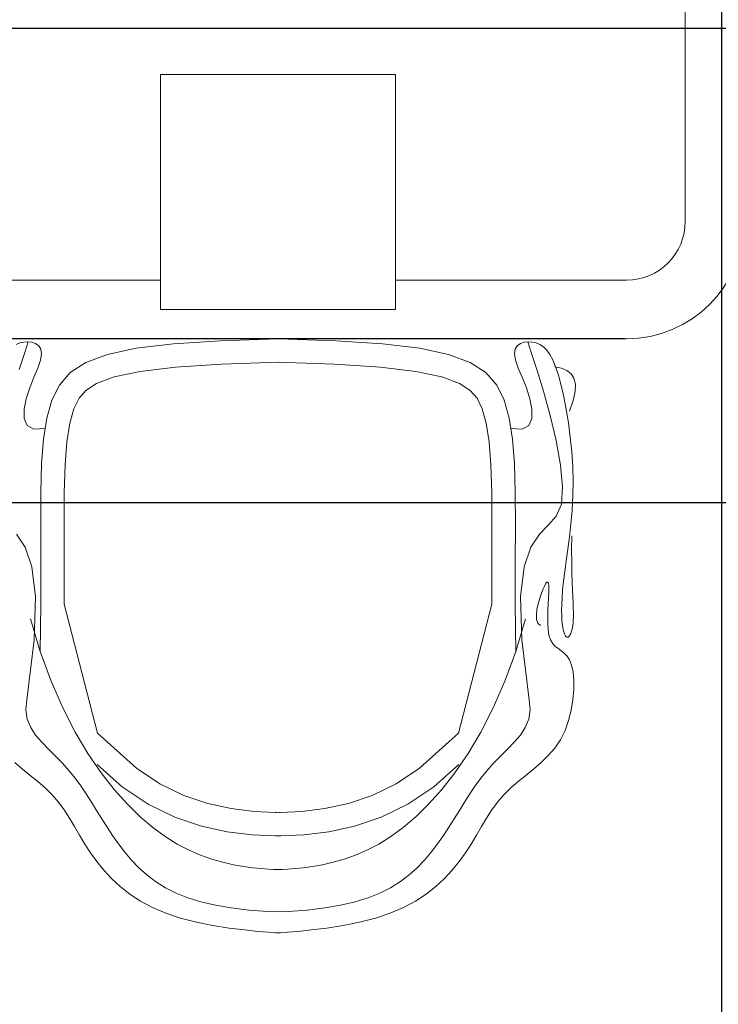
# Model space of a CAD drawing. Units: inches. Extents: x 1454 to 2136, y 626 to 1213.
# Tile 14 of 23: x 1678 to 1701, y 1062 to 1095. Entities that reach past the tile are written whole.
import ezdxf

# ---------------------------------------------------------------- set-up
doc = ezdxf.new("R2010")
doc.units = ezdxf.units.IN
doc.header["$MEASUREMENT"] = 0
for name, color, linetype, lineweight in [('A-ANNO-DIMS', 2, 'Continuous', 18), ('A-FURN-PATT', 252, 'Continuous', 13), ('conference', 41, 'Continuous', 18)]:
    doc.layers.add(name, color=color, linetype=linetype, lineweight=lineweight)
doc.styles.get("Standard").update_dxf_attribs({"font": 'arial.ttf'})
doc.dimstyles.get("Standard").update_dxf_attribs({"dimtxt": 4, "dimasz": 0.18, "dimexe": 0.18, "dimexo": 0.0625, "dimgap": 0.09, "dimtad": 0, "dimtih": 1, "dimtoh": 1, "dimdec": 0, "dimrnd": 6, "dimzin": 0, "dimdsep": 46, "dimlunit": 3, "dimtxsty": 'Standard', "dimcen": 0.09, "dimadec": 0, "dimazin": 0, "dimtfac": 1, "dimtdec": 0, "dimtofl": 0, "dimtmove": 0, "dimatfit": 3, "dimfxl": 1, "dimtolj": 1, "dimtzin": 0, "dimarcsym": 0})

# ---------------------------------------------------------------- blocks, each defined once
blk = doc.blocks.new('ОГ52_на12персон_стол2800х900')
for p, q in [((1350, -270.68), (1350, -520.68)), ((903.37, -595.68), (903.37, -395.68)), ((903.37, -395.68), (1103.37, -395.68)), ((1103.37, -395.68), (1103.37, -595.68)), ((903.37, -570.68), (603.37, -570.68)), ((1300, -570.68), (1103.37, -570.68)), ((1103.37, -595.68), (903.37, -595.68)), ((-1300, -620.68), (1300, -620.68)), ((783.57, -624.18), (780.44, -625.46)), ((786.91, -623.45), (783.57, -624.18)), ((790.43, -623.21), (786.91, -623.45)), ((787.79, -632.32), (790.86, -623.25)), ((793.92, -623.54), (790.43, -623.21)), ((797.1, -624.59), (793.92, -623.54)), ((799.71, -626.5), (797.1, -624.59)), ((801.46, -629.41), (799.71, -626.5)), ((882.76, -628.66), (914.4, -624.84)), ((914.4, -624.84), (954.25, -622.24)), ((954.25, -622.24), (1003.37, -620.68)), ((1052.48, -622.24), (1003.37, -620.68)), ((1092.33, -624.84), (1052.48, -622.24)), ((1123.97, -628.66), (1092.33, -624.84)), ((1205.28, -629.41), (1207.03, -626.5)), ((1207.03, -626.5), (1209.63, -624.59)), ((1209.63, -624.59), (1212.81, -623.54)), ((1212.81, -623.54), (1216.3, -623.21)), ((1218.94, -632.32), (1215.88, -623.25)), ((1216.3, -623.21), (1219.83, -623.45)), ((1219.83, -623.45), (1223.17, -624.18)), ((1223.17, -624.18), (1226.3, -625.46)), ((1226.3, -625.46), (1229.24, -627.43)), ((1229.24, -627.43), (1232.02, -630.19)), ((783.1, -646.8), (787.79, -632.32)), ((801.33, -638.81), (802.09, -633.47)), ((802.09, -633.47), (801.46, -629.41)), ((839.9, -640.74), (858.28, -633.9)), ((858.28, -633.9), (882.76, -628.66)), ((1148.45, -633.9), (1123.97, -628.66)), ((1166.83, -640.74), (1148.45, -633.9)), ((1204.65, -633.47), (1205.28, -629.41)), ((1205.41, -638.81), (1204.65, -633.47)), ((1223.64, -646.8), (1218.94, -632.32)), ((1232.02, -630.19), (1234.67, -633.88)), ((1234.67, -633.88), (1237.21, -638.62)), ((798.9, -645.58), (801.33, -638.81)), ((826.58, -649.4), (839.9, -640.74)), ((886.06, -648.4), (916.25, -644.76)), ((916.25, -644.76), (955.22, -642.22)), ((955.22, -642.22), (1004, -640.67)), ((1051.51, -642.22), (1002.73, -640.67)), ((1090.48, -644.76), (1051.51, -642.22)), ((1120.68, -648.4), (1090.48, -644.76)), ((1180.15, -649.4), (1166.83, -640.74)), ((1207.83, -645.58), (1205.41, -638.81)), ((1237.21, -638.62), (1239.66, -644.52)), ((1244.55, -645.63), (1239.08, -644.46)), ((1239.66, -644.52), (1242.06, -651.71)), ((795.53, -653.36), (792.03, -662.32)), ((798.9, -645.58), (795.53, -653.36)), ((817.26, -660.04), (826.58, -649.4)), ((848.95, -658.72), (863.89, -653.15)), ((863.89, -653.15), (886.06, -648.4)), ((1142.84, -653.15), (1120.68, -648.4)), ((1157.78, -658.72), (1142.84, -653.15)), ((1189.48, -660.04), (1180.15, -649.4)), ((1207.83, -645.58), (1211.21, -653.36)), ((1211.21, -653.36), (1214.71, -662.32)), ((1229.22, -665.14), (1223.64, -646.8)), ((1242.06, -651.71), (1244.4, -660.26)), ((1249.16, -647.56), (1244.55, -645.63)), ((1252.77, -650.38), (1249.16, -647.56)), ((1255.26, -654.22), (1252.77, -650.38)), ((810.88, -672.88), (817.26, -660.04)), ((839.8, -664.66), (848.95, -658.72)), ((1166.94, -664.66), (1157.78, -658.72)), ((1195.85, -672.88), (1189.48, -660.04)), ((1244.4, -660.26), (1246.64, -670.01)), ((1256.5, -659.21), (1255.26, -654.22)), ((1256.34, -665.48), (1256.5, -659.21)), ((792.03, -662.32), (789.06, -671.68)), ((834.02, -671.26), (839.8, -664.66)), ((1172.72, -671.26), (1166.94, -664.66)), ((1214.71, -662.32), (1217.68, -671.68)), ((1234.96, -685.83), (1229.22, -665.14)), ((1246.64, -670.01), (1248.73, -680.76)), ((1254.67, -673.16), (1256.34, -665.48)), ((789.06, -671.68), (787.28, -680.65)), ((806.53, -688.12), (810.88, -672.88)), ((829.61, -680.14), (834.02, -671.26)), ((1177.13, -680.14), (1172.72, -671.26)), ((1200.21, -688.12), (1195.85, -672.88)), ((1217.68, -671.68), (1219.46, -680.65)), ((1251.36, -682.38), (1254.67, -673.16)), ((787.28, -680.65), (787.33, -688.46)), ((826.1, -692.42), (829.61, -680.14)), ((1180.64, -692.42), (1177.13, -680.14)), ((1219.46, -680.65), (1219.4, -688.46)), ((1240.09, -707.33), (1234.96, -685.83)), ((1248.73, -680.76), (1250.58, -692.29)), ((787.33, -688.46), (789.89, -694.32)), ((789.89, -694.32), (795.6, -697.45)), ((803.73, -706.03), (806.53, -688.12)), ((823.61, -708.33), (826.1, -692.42)), ((1183.12, -708.33), (1180.64, -692.42)), ((1203.01, -706.03), (1200.21, -688.12)), ((1216.84, -694.32), (1211.13, -697.45)), ((1219.4, -688.46), (1216.84, -694.32)), ((1250.58, -692.29), (1252.14, -704.4)), ((795.6, -697.45), (805.13, -697.07)), ((1211.13, -697.45), (1201.61, -697.07)), ((802.16, -726.94), (803.73, -706.03)), ((822.14, -727.97), (823.61, -708.33)), ((1184.6, -727.97), (1183.12, -708.33)), ((1204.57, -726.94), (1203.01, -706.03)), ((1243.89, -728.11), (1240.09, -707.33)), ((1252.14, -704.4), (1253.35, -716.88)), ((1253.35, -716.88), (1254.14, -729.52)), ((801.49, -751.13), (802.16, -726.94)), ((821.48, -751.45), (822.14, -727.97)), ((1185.25, -751.45), (1184.6, -727.97)), ((1205.25, -751.13), (1204.57, -726.94)), ((1245.62, -746.63), (1243.89, -728.11)), ((1254.14, -729.52), (1254.45, -742.11)), ((1254.45, -742.11), (1254.24, -754.46)), ((801.37, -778.91), (801.49, -751.13)), ((821.37, -778.91), (821.48, -751.45)), ((1185.37, -778.91), (1185.25, -751.45)), ((1205.37, -778.91), (1205.25, -751.13)), ((1244.53, -761.38), (1245.62, -746.63)), ((1240.21, -771.53), (1244.53, -761.38)), ((1254.24, -754.46), (1253.59, -766.48)), ((1253.59, -766.48), (1252.6, -778.08)), ((801.48, -810.58), (801.37, -778.91)), ((821.48, -810.54), (821.37, -778.91)), ((1185.26, -810.54), (1185.37, -778.91)), ((1205.26, -810.58), (1205.37, -778.91)), ((1225.99, -787.04), (1233.61, -779.15)), ((1233.61, -779.15), (1240.21, -771.53)), ((1252.6, -778.08), (1251.38, -789.18)), ((788.11, -797.97), (780.75, -787.04)), ((1218.62, -797.97), (1225.99, -787.04)), ((1251.38, -789.18), (1250.05, -799.7)), ((1253.27, -800.21), (1253.41, -788.46)), ((793.95, -814.73), (788.11, -797.97)), ((1212.78, -814.73), (1218.62, -797.97)), ((1250.05, -799.7), (1248.69, -809.56)), ((1253.29, -810.55), (1253.27, -800.21)), ((801.48, -846.44), (801.48, -810.58)), ((821.48, -846.55), (821.48, -810.54)), ((1185.26, -846.55), (1185.26, -810.54)), ((1205.26, -846.44), (1205.26, -810.58)), ((1248.69, -809.56), (1247.43, -818.69)), ((1253.43, -819.6), (1253.29, -810.55)), ((796.99, -840.11), (793.95, -814.73)), ((1209.75, -840.11), (1212.78, -814.73)), ((1247.43, -818.69), (1246.37, -826.99)), ((1253.66, -827.5), (1253.43, -819.6)), ((1230.32, -830.57), (1231.41, -828.7)), ((1231.41, -828.7), (1232.29, -827.76)), ((1232.29, -827.76), (1232.98, -827.75)), ((1232.98, -827.75), (1233.48, -828.65)), ((1233.48, -828.65), (1233.79, -830.45)), ((1246.37, -826.99), (1245.58, -834.42)), ((1253.93, -834.35), (1253.66, -827.5)), ((1226.07, -841.47), (1227.56, -837.1)), ((1227.56, -837.1), (1229.03, -833.39)), ((1229.03, -833.39), (1230.32, -830.57)), ((1233.87, -836.73), (1233.66, -841.16)), ((1233.79, -830.45), (1233.92, -833.15)), ((1233.92, -833.15), (1233.87, -836.73)), ((1245.58, -834.42), (1245.06, -841)), ((1254.21, -840.27), (1253.93, -834.35)), ((795.96, -876.9), (796.99, -840.11)), ((801.03, -886.8), (801.48, -846.44)), ((849.76, -956.38), (821.48, -846.55)), ((1156.98, -956.38), (1185.26, -846.55)), ((1205.7, -886.8), (1205.26, -846.44)), ((1210.78, -876.9), (1209.75, -840.11)), ((1223.74, -850.99), (1224.74, -846.2)), ((1224.74, -846.2), (1226.07, -841.47)), ((1233.37, -846.22), (1233.09, -851.69)), ((1233.66, -841.16), (1233.37, -846.22)), ((1245.06, -841), (1244.78, -846.8)), ((1254.46, -845.39), (1254.21, -840.27)), ((1254.65, -849.83), (1254.46, -845.39)), ((1223.26, -855.54), (1223.74, -850.99)), ((1233.09, -851.69), (1232.92, -857.33)), ((1244.78, -846.8), (1244.7, -851.87)), ((1244.7, -851.87), (1244.79, -856.27)), ((1254.73, -853.68), (1254.65, -849.83)), ((1254.73, -857.02), (1254.73, -853.68)), ((792.73, -858.96), (801.02, -886.79)), ((1214, -858.96), (1205.72, -886.79)), ((1223.49, -859.55), (1223.26, -855.54)), ((1224.61, -862.74), (1223.49, -859.55)), ((1226.8, -864.79), (1224.61, -862.74)), ((1232.92, -857.33), (1232.95, -862.89)), ((1232.95, -862.89), (1233.27, -868.16)), ((1244.79, -856.27), (1245.01, -860.06)), ((1245.01, -860.06), (1245.34, -863.29)), ((1245.34, -863.29), (1245.73, -866.03)), ((1254.25, -864.48), (1254.47, -862.37)), ((1254.47, -862.37), (1254.64, -859.89)), ((1254.64, -859.89), (1254.73, -857.02)), ((1233.27, -868.16), (1233.98, -872.89)), ((1245.73, -866.03), (1246.17, -868.32)), ((1246.17, -868.32), (1246.63, -870.2)), ((1246.63, -870.2), (1247.12, -871.7)), ((1247.12, -871.7), (1247.62, -872.86)), ((1252.07, -872.49), (1252.5, -871.56)), ((1252.5, -871.56), (1252.9, -870.47)), ((1252.9, -870.47), (1253.28, -869.25)), ((1253.28, -869.25), (1253.64, -867.87)), ((1253.64, -867.87), (1253.97, -866.3)), ((1253.97, -866.3), (1254.25, -864.48)), ((789.59, -927.87), (795.96, -876.9)), ((1217.15, -927.87), (1210.78, -876.9)), ((1233.98, -872.89), (1235.17, -876.84)), ((1235.17, -876.84), (1236.9, -879.87)), ((1236.9, -879.87), (1239.07, -882.2)), ((1247.62, -872.86), (1248.14, -873.71)), ((1248.14, -873.71), (1248.66, -874.27)), ((1248.66, -874.27), (1249.18, -874.59)), ((1249.18, -874.59), (1249.7, -874.69)), ((1249.7, -874.69), (1250.2, -874.6)), ((1250.2, -874.6), (1250.69, -874.32)), ((1250.69, -874.32), (1251.17, -873.88)), ((1251.17, -873.88), (1251.63, -873.27)), ((1251.63, -873.27), (1252.07, -872.49)), ((801.02, -886.79), (810.21, -912.08)), ((1205.72, -886.79), (1196.52, -912.08)), ((1239.07, -882.2), (1241.52, -884.13)), ((1241.52, -884.13), (1244.12, -885.97)), ((1244.12, -885.97), (1246.74, -888.03)), ((1246.74, -888.03), (1249.22, -890.62)), ((1249.22, -890.62), (1251.43, -894.03)), ((1251.43, -894.03), (1253.22, -898.59)), ((1253.22, -898.59), (1254.46, -904.49)), ((1254.46, -904.49), (1255.11, -911.55)), ((810.21, -912.08), (820.14, -934.93)), ((1196.52, -912.08), (1186.59, -934.93)), ((1255.11, -911.55), (1255.1, -919.48)), ((1255.1, -919.48), (1254.4, -927.99)), ((789.59, -927.87), (788.79, -936.53)), ((1217.15, -927.87), (1217.95, -936.53)), ((1254.4, -927.99), (1252.96, -936.78)), ((788.79, -936.53), (790.01, -944.33)), ((820.14, -934.93), (830.65, -955.46)), ((1186.59, -934.93), (1176.08, -955.46)), ((1217.95, -936.53), (1216.73, -944.33)), ((1252.96, -936.78), (1250.73, -945.57)), ((790.01, -944.33), (792.9, -951.42)), ((1216.73, -944.33), (1213.84, -951.42)), ((1250.73, -945.57), (1247.67, -954.07)), ((792.9, -951.42), (797.11, -957.97)), ((830.65, -955.46), (841.58, -973.79)), ((1176.08, -955.46), (1165.16, -973.79)), ((1213.84, -951.42), (1209.63, -957.97)), ((1247.67, -954.07), (1243.73, -961.98)), ((797.11, -957.97), (802.27, -964.14)), ((849.76, -956.38), (883.04, -986.28)), ((1156.98, -956.38), (1123.7, -986.28)), ((1209.63, -957.97), (1204.47, -964.14)), ((1243.73, -961.98), (1238.91, -969.1)), ((802.27, -964.14), (808.04, -970.09)), ((808.04, -970.09), (814.05, -975.98)), ((1198.7, -970.09), (1192.68, -975.98)), ((1204.47, -964.14), (1198.7, -970.09)), ((1238.91, -969.1), (1233.35, -975.52)), ((814.05, -975.98), (819.96, -981.97)), ((841.58, -973.79), (852.75, -990.05)), ((1165.16, -973.79), (1153.98, -990.05)), ((1192.68, -975.98), (1186.78, -981.97)), ((1233.35, -975.52), (1227.26, -981.41)), ((779.47, -981.41), (785.91, -986.94)), ((785.91, -986.94), (792.49, -992.27)), ((819.96, -981.97), (825.48, -988.18)), ((825.48, -988.18), (830.62, -994.63)), ((849.41, -982.95), (870.75, -1002.12)), ((883.04, -986.28), (902.91, -999.52)), ((1123.7, -986.28), (1103.83, -999.52)), ((1157.33, -982.95), (1135.99, -1002.12)), ((1181.26, -988.18), (1176.12, -994.63)), ((1186.78, -981.97), (1181.26, -988.18)), ((1220.83, -986.94), (1214.25, -992.27)), ((1227.26, -981.41), (1220.83, -986.94)), ((792.49, -992.27), (799.02, -997.59)), ((830.62, -994.63), (835.45, -1001.27)), ((852.75, -990.05), (864.01, -1004.34)), ((1153.98, -990.05), (1142.73, -1004.34)), ((1176.12, -994.63), (1171.28, -1001.27)), ((1214.25, -992.27), (1207.71, -997.59)), ((799.02, -997.59), (805.32, -1003.05)), ((805.32, -1003.05), (811.18, -1008.83)), ((835.45, -1001.27), (840.06, -1008.08)), ((864.01, -1004.34), (875.19, -1016.78)), ((870.75, -1002.12), (892.96, -1016.92)), ((902.91, -999.52), (923.17, -1009.34)), ((1103.83, -999.52), (1083.56, -1009.34)), ((1135.99, -1002.12), (1113.78, -1016.92)), ((1142.73, -1004.34), (1131.55, -1016.78)), ((1171.28, -1001.27), (1166.67, -1008.08)), ((1201.42, -1003.05), (1195.56, -1008.83)), ((1207.71, -997.59), (1201.42, -1003.05)), ((811.18, -1008.83), (816.47, -1015.06)), ((840.06, -1008.08), (844.54, -1015.03)), ((923.17, -1009.34), (943.52, -1016.23)), ((1083.56, -1009.34), (1063.22, -1016.23)), ((1166.67, -1008.08), (1162.2, -1015.03)), ((1195.56, -1008.83), (1190.26, -1015.06)), ((816.47, -1015.06), (821.29, -1021.69)), ((821.29, -1021.69), (825.8, -1028.66)), ((844.54, -1015.03), (848.95, -1022.08)), ((848.95, -1022.08), (853.38, -1029.21)), ((875.19, -1016.78), (886.15, -1027.51)), ((892.96, -1016.92), (915.58, -1027.88)), ((943.52, -1016.23), (963.59, -1020.64)), ((963.59, -1020.64), (982.99, -1023.02)), ((1043.14, -1020.64), (1023.75, -1023.02)), ((1063.22, -1016.23), (1043.14, -1020.64)), ((1113.78, -1016.92), (1091.16, -1027.88)), ((1131.55, -1016.78), (1120.58, -1027.51)), ((1157.79, -1022.08), (1153.36, -1029.21)), ((1162.2, -1015.03), (1157.79, -1022.08)), ((1185.44, -1021.69), (1180.94, -1028.66)), ((1190.26, -1015.06), (1185.44, -1021.69)), ((825.8, -1028.66), (830.15, -1035.88)), ((853.38, -1029.21), (857.9, -1036.39)), ((886.15, -1027.51), (896.87, -1036.65)), ((915.58, -1027.88), (938.15, -1035.52)), ((982.99, -1023.02), (1001.26, -1023.82)), ((1001.26, -1023.82), (1002.98, -1023.78)), ((1005.48, -1023.82), (1003.76, -1023.78)), ((1023.75, -1023.02), (1005.48, -1023.82)), ((1091.16, -1027.88), (1068.59, -1035.52)), ((1120.58, -1027.51), (1109.86, -1036.65)), ((1153.36, -1029.21), (1148.83, -1036.39)), ((1180.94, -1028.66), (1176.58, -1035.88)), ((830.15, -1035.88), (834.5, -1043.27)), ((857.9, -1036.39), (862.61, -1043.58)), ((896.87, -1036.65), (907.36, -1044.36)), ((938.15, -1035.52), (960.22, -1040.38)), ((1068.59, -1035.52), (1046.52, -1040.38)), ((1109.86, -1036.65), (1099.37, -1044.36)), ((1148.83, -1036.39), (1144.13, -1043.58)), ((1176.58, -1035.88), (1172.23, -1043.27)), ((834.5, -1043.27), (839.01, -1050.76)), ((862.61, -1043.58), (867.57, -1050.71)), ((907.36, -1044.36), (917.61, -1050.77)), ((960.22, -1040.38), (981.33, -1042.97)), ((981.33, -1042.97), (1001.02, -1043.83)), ((1001.02, -1043.83), (1003.37, -1043.78)), ((1005.72, -1043.83), (1003.37, -1043.78)), ((1025.41, -1042.97), (1005.72, -1043.83)), ((1046.52, -1040.38), (1025.41, -1042.97)), ((1099.37, -1044.36), (1089.12, -1050.77)), ((1144.13, -1043.58), (1139.16, -1050.71)), ((1172.23, -1043.27), (1167.73, -1050.76)), ((839.01, -1050.76), (843.83, -1058.27)), ((867.57, -1050.71), (872.88, -1057.7)), ((917.61, -1050.77), (927.64, -1056.02)), ((927.64, -1056.02), (937.43, -1060.26)), ((1079.1, -1056.02), (1069.31, -1060.26)), ((1089.12, -1050.77), (1079.1, -1056.02)), ((1139.16, -1050.71), (1133.85, -1057.7)), ((1167.73, -1050.76), (1162.91, -1058.27)), ((843.83, -1058.27), (849.12, -1065.72)), ((872.88, -1057.7), (878.62, -1064.48)), ((878.62, -1064.48), (884.87, -1070.97)), ((937.43, -1060.26), (947, -1063.63)), ((947, -1063.63), (956.35, -1066.28)), ((1059.74, -1063.63), (1050.39, -1066.28)), ((1069.31, -1060.26), (1059.74, -1063.63)), ((1128.11, -1064.48), (1121.86, -1070.97)), ((1133.85, -1057.7), (1128.11, -1064.48)), ((1162.91, -1058.27), (1157.61, -1065.72)), ((849.12, -1065.72), (855.03, -1073.02)), ((884.87, -1070.97), (891.71, -1077.1)), ((956.35, -1066.28), (965.43, -1068.34)), ((965.43, -1068.34), (974.07, -1069.88)), ((974.07, -1069.88), (982.02, -1070.98)), ((982.02, -1070.98), (989.06, -1071.72)), ((989.06, -1071.72), (994.94, -1072.17)), ((994.94, -1072.17), (999.45, -1072.4)), ((999.45, -1072.4), (1002.33, -1072.49)), ((1002.33, -1072.49), (1003.37, -1072.5)), ((1004.4, -1072.49), (1003.37, -1072.5)), ((1007.29, -1072.4), (1004.4, -1072.49)), ((1011.79, -1072.17), (1007.29, -1072.4)), ((1017.68, -1071.72), (1011.79, -1072.17)), ((1024.71, -1070.98), (1017.68, -1071.72)), ((1032.66, -1069.88), (1024.71, -1070.98)), ((1041.3, -1068.34), (1032.66, -1069.88)), ((1050.39, -1066.28), (1041.3, -1068.34)), ((1121.86, -1070.97), (1115.02, -1077.1)), ((1157.61, -1065.72), (1151.71, -1073.02)), ((855.03, -1073.02), (861.64, -1080.11)), ((861.64, -1080.11), (869.03, -1086.91)), ((891.71, -1077.1), (899.23, -1082.79)), ((1115.02, -1077.1), (1107.5, -1082.79)), ((1145.1, -1080.11), (1137.71, -1086.91)), ((1151.71, -1073.02), (1145.1, -1080.11)), ((869.03, -1086.91), (877.28, -1093.35)), ((899.23, -1082.79), (907.51, -1087.97)), ((907.51, -1087.97), (916.64, -1092.56)), ((1099.22, -1087.97), (1090.1, -1092.56)), ((1107.5, -1082.79), (1099.22, -1087.97)), ((1137.71, -1086.91), (1129.46, -1093.35)), ((877.28, -1093.35), (886.46, -1099.33)), ((916.64, -1092.56), (926.71, -1096.58)), ((926.71, -1096.58), (937.82, -1100.01)), ((1080.03, -1096.58), (1068.92, -1100.01)), ((1090.1, -1092.56), (1080.03, -1096.58)), ((1129.46, -1093.35), (1120.28, -1099.33)), ((886.46, -1099.33), (896.65, -1104.8)), ((896.65, -1104.8), (907.92, -1109.67)), ((937.82, -1100.01), (950.08, -1102.88)), ((950.08, -1102.88), (963.59, -1105.18)), ((963.59, -1105.18), (978.44, -1106.93)), ((1043.15, -1105.18), (1028.29, -1106.93)), ((1056.66, -1102.88), (1043.15, -1105.18)), ((1068.92, -1100.01), (1056.66, -1102.88)), ((1110.09, -1104.8), (1098.81, -1109.67)), ((1120.28, -1099.33), (1110.09, -1104.8)), ((907.92, -1109.67), (920.36, -1113.86)), ((920.36, -1113.86), (933.9, -1117.34)), ((978.44, -1106.93), (994.75, -1108.13)), ((994.75, -1108.13), (1003.37, -1108.44)), ((1011.98, -1108.13), (1003.37, -1108.44)), ((1028.29, -1106.93), (1011.98, -1108.13)), ((1086.38, -1113.86), (1072.83, -1117.34)), ((1098.81, -1109.67), (1086.38, -1113.86)), ((933.9, -1117.34), (947.97, -1120.12)), ((947.97, -1120.12), (961.84, -1122.3)), ((961.84, -1122.3), (974.82, -1123.93)), ((1044.89, -1122.3), (1031.92, -1123.93)), ((1058.77, -1120.12), (1044.89, -1122.3)), ((1072.83, -1117.34), (1058.77, -1120.12)), ((974.82, -1123.93), (986.17, -1125.08)), ((986.17, -1125.08), (995.19, -1125.82)), ((995.19, -1125.82), (1001.16, -1126.21)), ((1001.16, -1126.21), (1003.37, -1126.33)), ((1005.58, -1126.21), (1003.37, -1126.33)), ((1011.55, -1125.82), (1005.58, -1126.21)), ((1020.57, -1125.08), (1011.55, -1125.82)), ((1031.92, -1123.93), (1020.57, -1125.08))]:
    blk.add_line(p, q)
for radius in [100, 50]:
    blk.add_arc((1300, -520.68), radius, 270, 0)
blk = doc.blocks.new('*D33')
at = {"layer": 'A-ANNO-DIMS', "color": 0, "lineweight": -2, "transparency": 16777216}
for p, q in [((2032.494, 1126.282), (1462.374, 1126.282)), ((1462.554, 1126.102), (1462.554, 1056.381)), ((1462.554, 982.462), (1462.554, 1052.184)), ((2032.494, 982.282), (1462.374, 982.282))]:
    blk.add_line(p, q, dxfattribs=at)
at = {"layer": 'A-ANNO-DIMS', "color": 0, "transparency": 16777216}
for points in [[(1462.524, 1126.102), (1462.584, 1126.102), (1462.554, 1126.282)], [(1462.524, 982.462), (1462.584, 982.462), (1462.554, 982.282)]]:
    blk.add_solid(points, dxfattribs=at)
at = {"layer": 'Defpoints', "color": 0, "transparency": 16777216}
for p in [(1462.554, 1126.282), (2032.556, 1126.282), (2032.556, 982.282)]:
    blk.add_point(p, dxfattribs=at)
at = {"layer": 'A-ANNO-DIMS', "color": 0, "transparency": 16777216, "insert": (1462.554, 1054.282), "char_height": 4, "attachment_point": 5}
blk.add_mtext('\\A1;144', dxfattribs=at)
blk = doc.blocks.new('*D45')
at = {"layer": 'A-ANNO-DIMS', "color": 0, "lineweight": -2, "transparency": 16777216}
for p, q in [((1654.556, 913.345), (1654.556, 1210.464)), ((1701.076, 909.11), (1701.076, 1210.464)), ((1654.736, 1210.284), (1670.917, 1210.284)), ((1700.896, 1210.284), (1684.715, 1210.284))]:
    blk.add_line(p, q, dxfattribs=at)
at = {"layer": 'A-ANNO-DIMS', "color": 0, "transparency": 16777216}
for points in [[(1654.736, 1210.314), (1654.736, 1210.254), (1654.556, 1210.284)], [(1700.896, 1210.314), (1700.896, 1210.254), (1701.076, 1210.284)]]:
    blk.add_solid(points, dxfattribs=at)
at = {"layer": 'Defpoints', "color": 0, "transparency": 16777216}
for p in [(1701.076, 1210.284), (1654.556, 913.282), (1701.076, 909.048)]:
    blk.add_point(p, dxfattribs=at)
at = {"layer": 'A-ANNO-DIMS', "color": 0, "transparency": 16777216, "insert": (1677.816, 1210.284), "char_height": 4, "attachment_point": 5}
blk.add_mtext('\\A1;46.52', dxfattribs=at)
blk = doc.blocks.new('*D54')
at = {"layer": 'A-ANNO-DIMS', "color": 0, "lineweight": -2, "transparency": 16777216}
for p, q in [((1879.494, 1126.282), (1462.374, 1126.282)), ((1462.554, 1126.102), (1462.554, 1078.915)), ((1462.554, 1027.462), (1462.554, 1074.65)), ((1879.494, 1027.282), (1462.374, 1027.282))]:
    blk.add_line(p, q, dxfattribs=at)
at = {"layer": 'A-ANNO-DIMS', "color": 0, "transparency": 16777216}
for points in [[(1462.524, 1126.102), (1462.584, 1126.102), (1462.554, 1126.282)], [(1462.524, 1027.462), (1462.584, 1027.462), (1462.554, 1027.282)]]:
    blk.add_solid(points, dxfattribs=at)
at = {"layer": 'Defpoints', "color": 0, "transparency": 16777216}
for p in [(1879.556, 1126.282), (1462.554, 1027.282), (1879.556, 1027.282)]:
    blk.add_point(p, dxfattribs=at)
at = {"layer": 'A-ANNO-DIMS', "color": 0, "transparency": 16777216, "insert": (1462.554, 1076.782), "char_height": 4, "attachment_point": 5}
blk.add_mtext('\\A1;99', dxfattribs=at)
blk = doc.blocks.new('*D68')
at = {"layer": 'A-ANNO-DIMS', "color": 0, "lineweight": -2, "transparency": 16777216}
for p, q in [((1659.724, 1027.329), (1659.724, 1210.464)), ((1704.308, 1027.329), (1704.308, 1210.464)), ((1659.904, 1210.284), (1675.092, 1210.284)), ((1704.128, 1210.284), (1688.939, 1210.284))]:
    blk.add_line(p, q, dxfattribs=at)
at = {"layer": 'A-ANNO-DIMS', "color": 0, "transparency": 16777216}
for points in [[(1659.904, 1210.314), (1659.904, 1210.254), (1659.724, 1210.284)], [(1704.128, 1210.314), (1704.128, 1210.254), (1704.308, 1210.284)]]:
    blk.add_solid(points, dxfattribs=at)
at = {"layer": 'Defpoints', "color": 0, "transparency": 16777216}
for p in [(1704.308, 1210.284), (1659.724, 1027.267), (1704.308, 1027.267)]:
    blk.add_point(p, dxfattribs=at)
at = {"layer": 'A-ANNO-DIMS', "color": 0, "transparency": 16777216, "insert": (1682.016, 1210.284), "char_height": 4, "attachment_point": 5}
blk.add_mtext('\\A1;44.58', dxfattribs=at)
blk = doc.blocks.new('*D70')
at = {"layer": 'A-ANNO-DIMS', "color": 0, "lineweight": -2, "transparency": 16777216}
for p, q in [((1811.166, 1094.525), (1462.374, 1094.525)), ((1462.554, 1094.345), (1462.554, 1088.71)), ((1462.554, 1078.811), (1462.554, 1084.445)), ((1811.166, 1078.631), (1462.374, 1078.631))]:
    blk.add_line(p, q, dxfattribs=at)
at = {"layer": 'A-ANNO-DIMS', "color": 0, "transparency": 16777216}
for points in [[(1462.524, 1094.345), (1462.584, 1094.345), (1462.554, 1094.525)], [(1462.524, 1078.811), (1462.584, 1078.811), (1462.554, 1078.631)]]:
    blk.add_solid(points, dxfattribs=at)
at = {"layer": 'Defpoints', "color": 0, "transparency": 16777216}
for p in [(1462.554, 1094.525), (1811.229, 1094.525), (1811.229, 1078.631)]:
    blk.add_point(p, dxfattribs=at)
at = {"layer": 'A-ANNO-DIMS', "color": 0, "transparency": 16777216, "insert": (1462.554, 1086.578), "char_height": 4, "attachment_point": 5}
blk.add_mtext('\\A1;15.894', dxfattribs=at)
blk = doc.blocks.new('*D76')
at = {"layer": 'A-ANNO-DIMS', "color": 0, "lineweight": -2, "transparency": 16777216}
for p, q in [((1962.644, 1095.65), (1462.374, 1095.65)), ((1462.554, 1095.47), (1462.554, 1073.782)), ((1462.554, 1047.83), (1462.554, 1069.517)), ((1914.644, 1047.65), (1462.374, 1047.65))]:
    blk.add_line(p, q, dxfattribs=at)
at = {"layer": 'A-ANNO-DIMS', "color": 0, "transparency": 16777216}
for points in [[(1462.524, 1095.47), (1462.584, 1095.47), (1462.554, 1095.65)], [(1462.524, 1047.83), (1462.584, 1047.83), (1462.554, 1047.65)]]:
    blk.add_solid(points, dxfattribs=at)
at = {"layer": 'Defpoints', "color": 0, "transparency": 16777216}
for p in [(1962.707, 1095.65), (1462.554, 1047.65), (1914.707, 1047.65)]:
    blk.add_point(p, dxfattribs=at)
at = {"layer": 'A-ANNO-DIMS', "color": 0, "transparency": 16777216, "insert": (1462.554, 1071.65), "char_height": 4, "attachment_point": 5}
blk.add_mtext('\\A1;48', dxfattribs=at)
blk = doc.blocks.new('*D82')
at = {"layer": 'A-ANNO-DIMS', "color": 0, "lineweight": -2, "transparency": 16777216}
for p, q in [((1697.818, 1084.129), (1462.374, 1084.129)), ((1462.554, 1083.949), (1462.554, 1057.83)), ((1462.554, 1027.447), (1462.554, 1053.565)), ((1704.245, 1027.267), (1462.374, 1027.267))]:
    blk.add_line(p, q, dxfattribs=at)
at = {"layer": 'A-ANNO-DIMS', "color": 0, "transparency": 16777216}
for points in [[(1462.524, 1083.949), (1462.584, 1083.949), (1462.554, 1084.129)], [(1462.524, 1027.447), (1462.584, 1027.447), (1462.554, 1027.267)]]:
    blk.add_solid(points, dxfattribs=at)
at = {"layer": 'Defpoints', "color": 0, "transparency": 16777216}
for p in [(1462.554, 1084.129), (1697.881, 1084.129), (1704.308, 1027.267)]:
    blk.add_point(p, dxfattribs=at)
at = {"layer": 'A-ANNO-DIMS', "color": 0, "transparency": 16777216, "insert": (1462.554, 1055.698), "char_height": 4, "attachment_point": 5}
blk.add_mtext('\\A1;56.86', dxfattribs=at)

msp = doc.modelspace()

# ---------------------------------------------------------------- hatches: boundary and pattern name
at = {"layer": 'A-FURN-PATT'}
h = msp.add_hatch(dxfattribs=at)
h.set_pattern_fill('ESCHER', color=256)
h.paths.add_polyline_path([(1511.3761, 923.7174, 1), (1525.379, 923.7174, 1)])
h.paths.add_polyline_path([(1525.379, 816.0542, 1), (1511.3761, 816.0542, 1)])
h.paths.add_polyline_path([(1525.379, 712.7345, 1), (1511.3761, 712.7345, 1)])
h.paths.add_polyline_path([(2070.5057, 794.3402, 1), (2056.5027, 794.3402, 1)])
h.paths.add_polyline_path([(2005.868, 1014.5578, 1), (1991.8651, 1014.5578, 1)])
h.paths.add_polyline_path([(1994.0647, 1066.7584, 1), (2008.0677, 1066.7584, 1)])
h.paths.add_polyline_path([(1919.5492, 1065.3848, 1), (1933.5521, 1065.3848, 1)])
h.paths.add_polyline_path([(1936.8517, 1013.7336, 1), (1922.8488, 1013.7336, 1)])
h.paths.add_polyline_path([(1824.6062, 1109.1557, 1), (1838.6091, 1109.1557, 1)])

# ---------------------------------------------------------------- block references
at = {"layer": 'conference', "xscale": 0.0393700787401575, "yscale": 0.0393700787401575, "zscale": 0.0393700787401575}
msp.add_blockref('ОГ52_на12персон_стол2800х900', (1646.6996, 1108.5647), dxfattribs=at)

# ---------------------------------------------------------------- dimensions: what is measured, and where the dimension line sits
at = {"layer": 'A-ANNO-DIMS'}
for base, p1, p2, picture, middle in [((1701.0763, 1210.2845), (1654.5563, 913.2825), (1701.0763, 909.0476), '*D45', (1677.8163, 1210.2845)), ((1704.308, 1210.2845), (1659.7237, 1027.2667), (1704.308, 1027.2667), '*D68', (1682.0158, 1210.2845))]:
    dim = msp.add_linear_dim(base=base, p1=p1, p2=p2, dimstyle='Standard', override={"dimdec": 2, "dimlfac": 1, "dimrnd": 0, "dimzin": 0, "dimdsep": 46, "dimlunit": 2}, dxfattribs=at)
    dim.commit()
    dim.dimension.update_dxf_attribs({"geometry": picture, "text_midpoint": middle})
for base, p1, p2, override, picture, middle in [((1462.5543, 1126.2825), (2032.5563, 982.2825), (2032.5563, 1126.2825), {"dimdec": 0, "dimlfac": 1, "dimrnd": 0, "dimzin": 0, "dimdsep": 46, "dimlunit": 2}, '*D33', (1462.5543, 1054.2825)), ((1462.5543, 1027.2825), (1879.5563, 1126.2825), (1879.5563, 1027.2825), {"dimdec": 0, "dimlfac": 1, "dimrnd": 0, "dimzin": 0, "dimdsep": 46, "dimlunit": 2}, '*D54', (1462.5543, 1076.7825)), ((1462.5543, 1047.6495), (1962.7068, 1095.6495), (1914.7068, 1047.6495), {"dimdec": 0, "dimlfac": 1, "dimrnd": 0, "dimzin": 0, "dimdsep": 46, "dimlunit": 2}, '*D76', (1462.5543, 1071.6495)), ((1462.5543, 1094.5248), (1811.2288, 1078.6305), (1811.2288, 1094.5248), {"dimdec": 3, "dimlfac": 1, "dimrnd": 0, "dimzin": 0, "dimdsep": 46, "dimlunit": 2}, '*D70', (1462.5543, 1086.5777)), ((1462.5543, 1084.1285), (1704.308, 1027.2667), (1697.8807, 1084.1285), {"dimdec": 2, "dimlfac": 1, "dimrnd": 0, "dimzin": 0, "dimdsep": 46, "dimlunit": 2}, '*D82', (1462.5543, 1055.6976))]:
    dim = msp.add_linear_dim(base=base, p1=p1, p2=p2, angle=90, dimstyle='Standard', override=override, dxfattribs=at)
    dim.commit()
    dim.dimension.update_dxf_attribs({"geometry": picture, "text_midpoint": middle})

doc.saveas('drawing.dxf')
